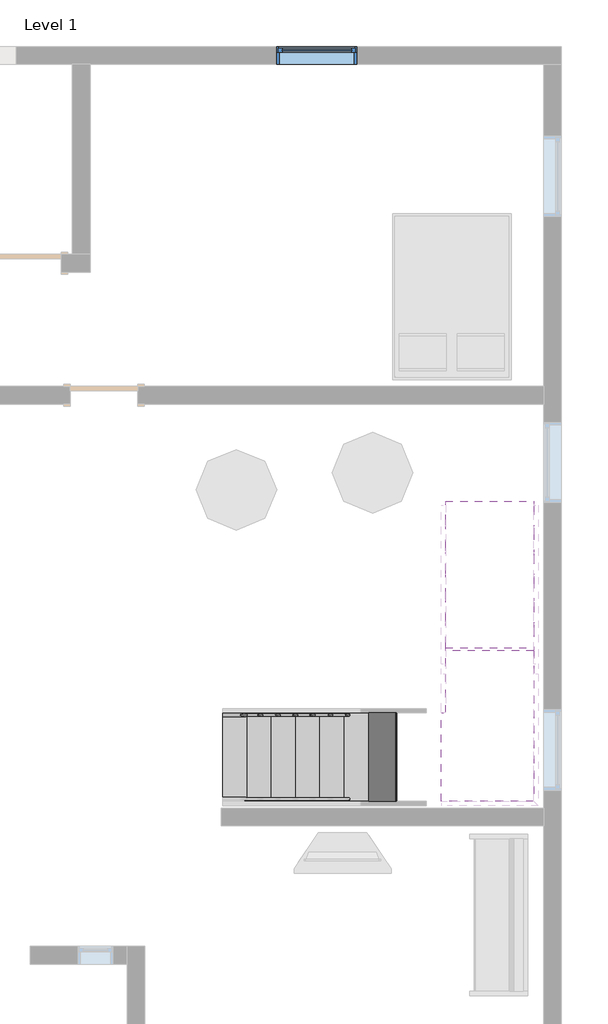
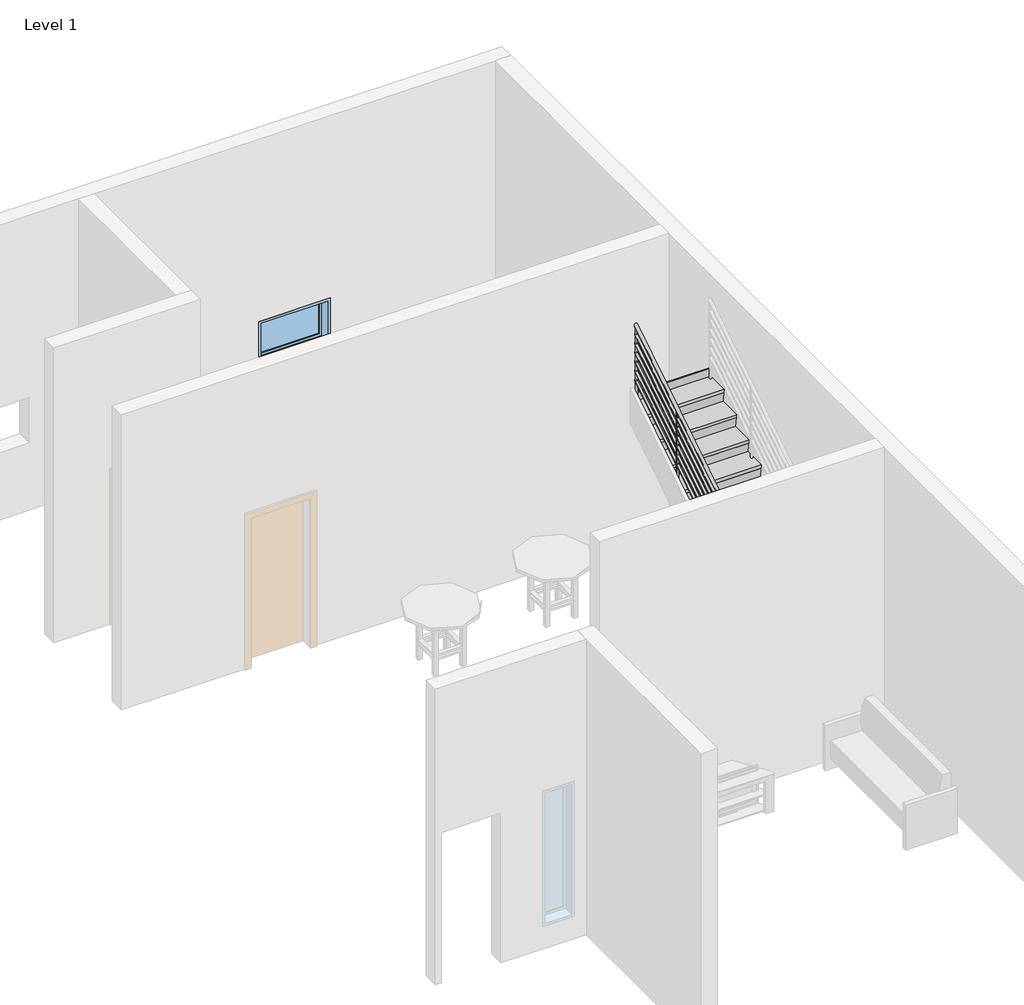
# One storey, part 2 of 4: 2 stair flights, 1 railing, 1 slab, 1 window.
"""IFC4 building model written with IfcOpenShell, lengths in millimetres."""

from ifc_helpers import new_model, si_unit, point, frame, frame_2d, origin, place, context, project, spatial, circle_curve, ellipse_curve, trimmed, segment, composite_curve, outline, extrude, transform, mapped, element, save
from ifc_brep_helpers import plane_surface, cylinder_surface, advanced_brep
from components import non_monolithic_landing_00e8e037, stair_flight_50mm_tread_25mm_nosing_13mm_riser_ecbb9275, stair_flight_50mm_tread_25mm_nosing_13mm_riser_0ce5104d, m_fixed_0915_x_0610mm_70a843a6

model = new_model("IFC4")

# Units and contexts
model_context = context("Model", 3, world=origin())
ifc_project = project(units=[si_unit("LENGTHUNIT", "METRE", prefix="MILLI")], contexts=[model_context])

# Site, building, storey
site = spatial("IfcSite", under=ifc_project)
building = spatial("IfcBuilding", under=site)
storey = spatial("IfcBuildingStorey", under=building, Name="Level 1", Elevation=0.0)

# Railing
placement = place(None, origin())
element("IfcRailing", 1, ObjectType="900mm Pipe", at=placement, inside=storey, context=model_context, shape_type="SolidModel", body=[
    advanced_brep(
    [(-399.786154, 3701.652048, 1050.2491997), (-399.786154, 3741.652048, 1050.2491997), (2081.007299, 3701.652048, 2619.1304348), (2081.007299, 3741.652048, 2619.1304348), (2171.413846, 3701.652048, 2619.1304348), (2131.413846, 3741.652048, 2619.1304348), (2171.413846, 4184.041917, 2619.1304348), (2131.413846, 4184.041917, 2619.1304348), (2171.413846, 6103.248464, 3832.8578953), (2131.413846, 6103.248464, 3832.8578953)],
    [
        (0, 1, ellipse_curve(frame((-399.786154, 3721.652048, 1050.2491997), z_axis=(-1.0, 0.0, 0.0), x_axis=(0.0, 0.0, -1.0)), 23.6638438, 20.0)),
        (1, 0, ellipse_curve(frame((-399.786154, 3721.652048, 1050.2491997), z_axis=(-1.0, 0.0, 0.0), x_axis=(0.0, 0.0, -1.0)), 23.6638438, 20.0)),
        (0, 2),
        (2, 3, ellipse_curve(frame((2081.007299, 3721.652048, 2619.1304348), z_axis=(-0.9605132043335073, 0.0, -0.27823440531497545), x_axis=(0.2782344053149749, 0.0, -0.9605132043335074)), 20.822202, 20.0)),
        (3, 1),
        (3, 2, ellipse_curve(frame((2081.007299, 3721.652048, 2619.1304348), z_axis=(-0.9605132043335073, 0.0, -0.27823440531497545), x_axis=(0.2782344053149749, 0.0, -0.9605132043335074)), 20.822202, 20.0)),
        (2, 4),
        (4, 5, ellipse_curve(frame((2151.413846, 3721.652048, 2619.1304348), z_axis=(-0.7071067811865482, -0.7071067811865468, 0.0), x_axis=(-0.7071067811865468, 0.7071067811865482, 0.0)), 28.2842712, 20.0)),
        (5, 3),
        (5, 4, ellipse_curve(frame((2151.413846, 3721.652048, 2619.1304348), z_axis=(-0.7071067811865482, -0.7071067811865468, 0.0), x_axis=(-0.7071067811865468, 0.7071067811865482, 0.0)), 28.2842712, 20.0)),
        (4, 6),
        (6, 7, ellipse_curve(frame((2151.413846, 4184.041917, 2619.1304348), z_axis=(0.0, -0.9605132043335073, -0.27823440531497556), x_axis=(0.0, -0.2782344053149757, 0.9605132043335073)), 20.822202, 20.0)),
        (7, 5),
        (7, 6, ellipse_curve(frame((2151.413846, 4184.041917, 2619.1304348), z_axis=(0.0, -0.9605132043335073, -0.27823440531497556), x_axis=(0.0, -0.2782344053149757, 0.9605132043335073)), 20.822202, 20.0)),
        (8, 9, ellipse_curve(frame((2151.413846, 6103.248464, 3832.8578953), z_axis=(0.0, 1.0, 0.0), x_axis=(0.0, 0.0, -1.0)), 23.6638438, 20.0)),
        (9, 8, ellipse_curve(frame((2151.413846, 6103.248464, 3832.8578953), z_axis=(0.0, 1.0, 0.0), x_axis=(0.0, 0.0, -1.0)), 23.6638438, 20.0)),
        (6, 8),
        (9, 7),
    ],
    [
        plane_surface(frame((-399.786154, 3721.652048, 1073.9130435), z_axis=(-1.0, 0.0, 0.0), x_axis=(0.0, 1.0, 0.0))),
        cylinder_surface(frame((-389.0962412, 3721.652048, 1057.0096189), z_axis=(-0.845171231398044, 0.0, -0.5344956404098299), x_axis=(0.0, 1.0, 0.0)), 20.0),
        cylinder_surface(frame((2075.213846, 3721.652048, 2619.1304348), z_axis=(-1.0, 0.0, 0.0), x_axis=(0.0, 1.0, 0.0)), 20.0),
        cylinder_surface(frame((2151.413846, 3721.652048, 2619.1304348), z_axis=(0.0, -1.0, 0.0), x_axis=(-1.0, 0.0, 0.0)), 20.0),
        plane_surface(frame((2151.413846, 6103.248464, 3856.5217391), z_axis=(0.0, 1.0, 0.0), x_axis=(0.0, 0.0, 1.0))),
        cylinder_surface(frame((2151.413846, 4188.9383768, 2622.2270102), z_axis=(0.0, -0.8451712313980438, -0.5344956404098301), x_axis=(-1.0, 0.0, 0.0)), 20.0),
    ],
    [
        (0, [[1, 2]]),
        (1, [[-1, 3, 4, 5]]),
        (1, [[-2, -5, 6, -3]]),
        (2, [[-4, 7, 8, 9]]),
        (2, [[-6, -9, 10, -7]]),
        (3, [[-8, 11, 12, 13]]),
        (3, [[-10, -13, 14, -11]]),
        (4, [[15, 16]]),
        (5, [[-12, 17, -16, 18]]),
        (5, [[-14, -18, -15, -17]]),
    ],
),
    advanced_brep(
    [(-399.786154, 3706.652048, 931.1651606), (-399.786154, 3736.652048, 931.1651606), (2079.5589357, 3706.652048, 2499.1304348), (2079.5589357, 3736.652048, 2499.1304348), (2166.413846, 3706.652048, 2499.1304348), (2136.413846, 3736.652048, 2499.1304348), (2166.413846, 4182.5935537, 2499.1304348), (2136.413846, 4182.5935537, 2499.1304348), (2166.413846, 6103.248464, 3713.7738563), (2136.413846, 6103.248464, 3713.7738563)],
    [
        (0, 1, ellipse_curve(frame((-399.786154, 3721.652048, 931.1651606), z_axis=(-1.0, 0.0, 0.0), x_axis=(0.0, 0.0, -1.0)), 17.7478828, 15.0)),
        (1, 0, ellipse_curve(frame((-399.786154, 3721.652048, 931.1651606), z_axis=(-1.0, 0.0, 0.0), x_axis=(0.0, 0.0, -1.0)), 17.7478828, 15.0)),
        (0, 2),
        (2, 3, ellipse_curve(frame((2079.5589357, 3721.652048, 2499.1304348), z_axis=(-0.9605132043335073, 0.0, -0.27823440531497545), x_axis=(0.2782344053149749, 0.0, -0.9605132043335074)), 15.6166515, 15.0)),
        (3, 1),
        (3, 2, ellipse_curve(frame((2079.5589357, 3721.652048, 2499.1304348), z_axis=(-0.9605132043335073, 0.0, -0.27823440531497545), x_axis=(0.2782344053149749, 0.0, -0.9605132043335074)), 15.6166515, 15.0)),
        (2, 4),
        (4, 5, ellipse_curve(frame((2151.413846, 3721.652048, 2499.1304348), z_axis=(-0.7071067811865482, -0.7071067811865468, 0.0), x_axis=(-0.7071067811865468, 0.7071067811865482, 0.0)), 21.2132034, 15.0)),
        (5, 3),
        (5, 4, ellipse_curve(frame((2151.413846, 3721.652048, 2499.1304348), z_axis=(-0.7071067811865482, -0.7071067811865468, 0.0), x_axis=(-0.7071067811865468, 0.7071067811865482, 0.0)), 21.2132034, 15.0)),
        (4, 6),
        (6, 7, ellipse_curve(frame((2151.413846, 4182.5935537, 2499.1304348), z_axis=(0.0, -0.9605132043335073, -0.27823440531497556), x_axis=(0.0, -0.2782344053149757, 0.9605132043335073)), 15.6166515, 15.0)),
        (7, 5),
        (7, 6, ellipse_curve(frame((2151.413846, 4182.5935537, 2499.1304348), z_axis=(0.0, -0.9605132043335073, -0.27823440531497556), x_axis=(0.0, -0.2782344053149757, 0.9605132043335073)), 15.6166515, 15.0)),
        (8, 9, ellipse_curve(frame((2151.413846, 6103.248464, 3713.7738563), z_axis=(0.0, 1.0, 0.0), x_axis=(0.0, 0.0, -1.0)), 17.7478828, 15.0)),
        (9, 8, ellipse_curve(frame((2151.413846, 6103.248464, 3713.7738563), z_axis=(0.0, 1.0, 0.0), x_axis=(0.0, 0.0, -1.0)), 17.7478828, 15.0)),
        (6, 8),
        (9, 7),
    ],
    [
        plane_surface(frame((-399.786154, 3721.652048, 948.9130435), z_axis=(-1.0, 0.0, 0.0), x_axis=(0.0, 1.0, 0.0))),
        cylinder_surface(frame((-391.7687194, 3721.652048, 936.235475), z_axis=(-0.845171231398044, 0.0, -0.5344956404098299), x_axis=(0.0, 1.0, 0.0)), 15.0),
        cylinder_surface(frame((2075.213846, 3721.652048, 2499.1304348), z_axis=(-1.0, 0.0, 0.0), x_axis=(0.0, 1.0, 0.0)), 15.0),
        cylinder_surface(frame((2151.413846, 3721.652048, 2499.1304348), z_axis=(0.0, -1.0, 0.0), x_axis=(-1.0, 0.0, 0.0)), 15.0),
        plane_surface(frame((2151.413846, 6103.248464, 3731.5217391), z_axis=(0.0, 1.0, 0.0), x_axis=(0.0, 0.0, 1.0))),
        cylinder_surface(frame((2151.413846, 4186.2658986, 2501.4528663), z_axis=(0.0, -0.8451712313980438, -0.5344956404098301), x_axis=(-1.0, 0.0, 0.0)), 15.0),
    ],
    [
        (0, [[1, 2]]),
        (1, [[-1, 3, 4, 5]]),
        (1, [[-2, -5, 6, -3]]),
        (2, [[-4, 7, 8, 9]]),
        (2, [[-6, -9, 10, -7]]),
        (3, [[-8, 11, 12, 13]]),
        (3, [[-10, -13, 14, -11]]),
        (4, [[15, 16]]),
        (5, [[-12, 17, -16, 18]]),
        (5, [[-14, -18, -15, -17]]),
    ],
),
    advanced_brep(
    [(-399.786154, 3706.652048, 806.1651606), (-399.786154, 3736.652048, 806.1651606), (2079.5589357, 3706.652048, 2374.1304348), (2079.5589357, 3736.652048, 2374.1304348), (2166.413846, 3706.652048, 2374.1304348), (2136.413846, 3736.652048, 2374.1304348), (2166.413846, 4182.5935537, 2374.1304348), (2136.413846, 4182.5935537, 2374.1304348), (2166.413846, 6103.248464, 3588.7738563), (2136.413846, 6103.248464, 3588.7738563)],
    [
        (0, 1, ellipse_curve(frame((-399.786154, 3721.652048, 806.1651606), z_axis=(-1.0, 0.0, 0.0), x_axis=(0.0, 0.0, -1.0)), 17.7478828, 15.0)),
        (1, 0, ellipse_curve(frame((-399.786154, 3721.652048, 806.1651606), z_axis=(-1.0, 0.0, 0.0), x_axis=(0.0, 0.0, -1.0)), 17.7478828, 15.0)),
        (0, 2),
        (2, 3, ellipse_curve(frame((2079.5589357, 3721.652048, 2374.1304348), z_axis=(-0.9605132043335073, 0.0, -0.27823440531497545), x_axis=(0.2782344053149749, 0.0, -0.9605132043335074)), 15.6166515, 15.0)),
        (3, 1),
        (3, 2, ellipse_curve(frame((2079.5589357, 3721.652048, 2374.1304348), z_axis=(-0.9605132043335073, 0.0, -0.27823440531497545), x_axis=(0.2782344053149749, 0.0, -0.9605132043335074)), 15.6166515, 15.0)),
        (2, 4),
        (4, 5, ellipse_curve(frame((2151.413846, 3721.652048, 2374.1304348), z_axis=(-0.7071067811865482, -0.7071067811865468, 0.0), x_axis=(-0.7071067811865468, 0.7071067811865482, 0.0)), 21.2132034, 15.0)),
        (5, 3),
        (5, 4, ellipse_curve(frame((2151.413846, 3721.652048, 2374.1304348), z_axis=(-0.7071067811865482, -0.7071067811865468, 0.0), x_axis=(-0.7071067811865468, 0.7071067811865482, 0.0)), 21.2132034, 15.0)),
        (4, 6),
        (6, 7, ellipse_curve(frame((2151.413846, 4182.5935537, 2374.1304348), z_axis=(0.0, -0.9605132043335073, -0.27823440531497556), x_axis=(0.0, -0.2782344053149757, 0.9605132043335073)), 15.6166515, 15.0)),
        (7, 5),
        (7, 6, ellipse_curve(frame((2151.413846, 4182.5935537, 2374.1304348), z_axis=(0.0, -0.9605132043335073, -0.27823440531497556), x_axis=(0.0, -0.2782344053149757, 0.9605132043335073)), 15.6166515, 15.0)),
        (8, 9, ellipse_curve(frame((2151.413846, 6103.248464, 3588.7738563), z_axis=(0.0, 1.0, 0.0), x_axis=(0.0, 0.0, -1.0)), 17.7478828, 15.0)),
        (9, 8, ellipse_curve(frame((2151.413846, 6103.248464, 3588.7738563), z_axis=(0.0, 1.0, 0.0), x_axis=(0.0, 0.0, -1.0)), 17.7478828, 15.0)),
        (6, 8),
        (9, 7),
    ],
    [
        plane_surface(frame((-399.786154, 3721.652048, 823.9130435), z_axis=(-1.0, 0.0, 0.0), x_axis=(0.0, 1.0, 0.0))),
        cylinder_surface(frame((-391.7687194, 3721.652048, 811.235475), z_axis=(-0.845171231398044, 0.0, -0.5344956404098299), x_axis=(0.0, 1.0, 0.0)), 15.0),
        cylinder_surface(frame((2075.213846, 3721.652048, 2374.1304348), z_axis=(-1.0, 0.0, 0.0), x_axis=(0.0, 1.0, 0.0)), 15.0),
        cylinder_surface(frame((2151.413846, 3721.652048, 2374.1304348), z_axis=(0.0, -1.0, 0.0), x_axis=(-1.0, 0.0, 0.0)), 15.0),
        plane_surface(frame((2151.413846, 6103.248464, 3606.5217391), z_axis=(0.0, 1.0, 0.0), x_axis=(0.0, 0.0, 1.0))),
        cylinder_surface(frame((2151.413846, 4186.2658986, 2376.4528663), z_axis=(0.0, -0.8451712313980438, -0.5344956404098301), x_axis=(-1.0, 0.0, 0.0)), 15.0),
    ],
    [
        (0, [[1, 2]]),
        (1, [[-1, 3, 4, 5]]),
        (1, [[-2, -5, 6, -3]]),
        (2, [[-4, 7, 8, 9]]),
        (2, [[-6, -9, 10, -7]]),
        (3, [[-8, 11, 12, 13]]),
        (3, [[-10, -13, 14, -11]]),
        (4, [[15, 16]]),
        (5, [[-12, 17, -16, 18]]),
        (5, [[-14, -18, -15, -17]]),
    ],
),
    advanced_brep(
    [(-399.786154, 3706.652048, 681.1651606), (-399.786154, 3736.652048, 681.1651606), (2079.5589357, 3706.652048, 2249.1304348), (2079.5589357, 3736.652048, 2249.1304348), (2166.413846, 3706.652048, 2249.1304348), (2136.413846, 3736.652048, 2249.1304348), (2166.413846, 4182.5935537, 2249.1304348), (2136.413846, 4182.5935537, 2249.1304348), (2166.413846, 6103.248464, 3463.7738563), (2136.413846, 6103.248464, 3463.7738563)],
    [
        (0, 1, ellipse_curve(frame((-399.786154, 3721.652048, 681.1651606), z_axis=(-1.0, 0.0, 0.0), x_axis=(0.0, 0.0, -1.0)), 17.7478828, 15.0)),
        (1, 0, ellipse_curve(frame((-399.786154, 3721.652048, 681.1651606), z_axis=(-1.0, 0.0, 0.0), x_axis=(0.0, 0.0, -1.0)), 17.7478828, 15.0)),
        (0, 2),
        (2, 3, ellipse_curve(frame((2079.5589357, 3721.652048, 2249.1304348), z_axis=(-0.9605132043335073, 0.0, -0.27823440531497545), x_axis=(0.2782344053149749, 0.0, -0.9605132043335074)), 15.6166515, 15.0)),
        (3, 1),
        (3, 2, ellipse_curve(frame((2079.5589357, 3721.652048, 2249.1304348), z_axis=(-0.9605132043335073, 0.0, -0.27823440531497545), x_axis=(0.2782344053149749, 0.0, -0.9605132043335074)), 15.6166515, 15.0)),
        (2, 4),
        (4, 5, ellipse_curve(frame((2151.413846, 3721.652048, 2249.1304348), z_axis=(-0.7071067811865482, -0.7071067811865468, 0.0), x_axis=(-0.7071067811865468, 0.7071067811865482, 0.0)), 21.2132034, 15.0)),
        (5, 3),
        (5, 4, ellipse_curve(frame((2151.413846, 3721.652048, 2249.1304348), z_axis=(-0.7071067811865482, -0.7071067811865468, 0.0), x_axis=(-0.7071067811865468, 0.7071067811865482, 0.0)), 21.2132034, 15.0)),
        (4, 6),
        (6, 7, ellipse_curve(frame((2151.413846, 4182.5935537, 2249.1304348), z_axis=(0.0, -0.9605132043335073, -0.27823440531497545), x_axis=(0.0, -0.2782344053149758, 0.9605132043335072)), 15.6166515, 15.0)),
        (7, 5),
        (7, 6, ellipse_curve(frame((2151.413846, 4182.5935537, 2249.1304348), z_axis=(0.0, -0.9605132043335073, -0.27823440531497545), x_axis=(0.0, -0.2782344053149758, 0.9605132043335072)), 15.6166515, 15.0)),
        (8, 9, ellipse_curve(frame((2151.413846, 6103.248464, 3463.7738563), z_axis=(0.0, 1.0, 0.0), x_axis=(0.0, 0.0, -1.0)), 17.7478828, 15.0)),
        (9, 8, ellipse_curve(frame((2151.413846, 6103.248464, 3463.7738563), z_axis=(0.0, 1.0, 0.0), x_axis=(0.0, 0.0, -1.0)), 17.7478828, 15.0)),
        (6, 8),
        (9, 7),
    ],
    [
        plane_surface(frame((-399.786154, 3721.652048, 698.9130435), z_axis=(-1.0, 0.0, 0.0), x_axis=(0.0, 1.0, 0.0))),
        cylinder_surface(frame((-391.7687194, 3721.652048, 686.235475), z_axis=(-0.845171231398044, 0.0, -0.5344956404098299), x_axis=(0.0, 1.0, 0.0)), 15.0),
        cylinder_surface(frame((2075.213846, 3721.652048, 2249.1304348), z_axis=(-1.0, 0.0, 0.0), x_axis=(0.0, 1.0, 0.0)), 15.0),
        cylinder_surface(frame((2151.413846, 3721.652048, 2249.1304348), z_axis=(0.0, -1.0, 0.0), x_axis=(-1.0, 0.0, 0.0)), 15.0),
        plane_surface(frame((2151.413846, 6103.248464, 3481.5217391), z_axis=(0.0, 1.0, 0.0), x_axis=(0.0, 0.0, 1.0))),
        cylinder_surface(frame((2151.413846, 4186.2658986, 2251.4528663), z_axis=(0.0, -0.845171231398044, -0.5344956404098299), x_axis=(-1.0, 0.0, 0.0)), 15.0),
    ],
    [
        (0, [[1, 2]]),
        (1, [[-1, 3, 4, 5]]),
        (1, [[-2, -5, 6, -3]]),
        (2, [[-4, 7, 8, 9]]),
        (2, [[-6, -9, 10, -7]]),
        (3, [[-8, 11, 12, 13]]),
        (3, [[-10, -13, 14, -11]]),
        (4, [[15, 16]]),
        (5, [[-12, 17, -16, 18]]),
        (5, [[-14, -18, -15, -17]]),
    ],
),
    advanced_brep(
    [(-399.786154, 3706.652048, 556.1651606), (-399.786154, 3736.652048, 556.1651606), (2079.5589357, 3706.652048, 2124.1304348), (2079.5589357, 3736.652048, 2124.1304348), (2166.413846, 3706.652048, 2124.1304348), (2136.413846, 3736.652048, 2124.1304348), (2166.413846, 4182.5935537, 2124.1304348), (2136.413846, 4182.5935537, 2124.1304348), (2166.413846, 6103.248464, 3338.7738563), (2136.413846, 6103.248464, 3338.7738563)],
    [
        (0, 1, ellipse_curve(frame((-399.786154, 3721.652048, 556.1651606), z_axis=(-1.0, 0.0, 0.0), x_axis=(0.0, 0.0, -1.0)), 17.7478828, 15.0)),
        (1, 0, ellipse_curve(frame((-399.786154, 3721.652048, 556.1651606), z_axis=(-1.0, 0.0, 0.0), x_axis=(0.0, 0.0, -1.0)), 17.7478828, 15.0)),
        (0, 2),
        (2, 3, ellipse_curve(frame((2079.5589357, 3721.652048, 2124.1304348), z_axis=(-0.9605132043335073, 0.0, -0.27823440531497545), x_axis=(0.2782344053149749, 0.0, -0.9605132043335074)), 15.6166515, 15.0)),
        (3, 1),
        (3, 2, ellipse_curve(frame((2079.5589357, 3721.652048, 2124.1304348), z_axis=(-0.9605132043335073, 0.0, -0.27823440531497545), x_axis=(0.2782344053149749, 0.0, -0.9605132043335074)), 15.6166515, 15.0)),
        (2, 4),
        (4, 5, ellipse_curve(frame((2151.413846, 3721.652048, 2124.1304348), z_axis=(-0.7071067811865482, -0.7071067811865468, 0.0), x_axis=(-0.7071067811865468, 0.7071067811865482, 0.0)), 21.2132034, 15.0)),
        (5, 3),
        (5, 4, ellipse_curve(frame((2151.413846, 3721.652048, 2124.1304348), z_axis=(-0.7071067811865482, -0.7071067811865468, 0.0), x_axis=(-0.7071067811865468, 0.7071067811865482, 0.0)), 21.2132034, 15.0)),
        (4, 6),
        (6, 7, ellipse_curve(frame((2151.413846, 4182.5935537, 2124.1304348), z_axis=(0.0, -0.9605132043335073, -0.27823440531497556), x_axis=(0.0, -0.2782344053149757, 0.9605132043335073)), 15.6166515, 15.0)),
        (7, 5),
        (7, 6, ellipse_curve(frame((2151.413846, 4182.5935537, 2124.1304348), z_axis=(0.0, -0.9605132043335073, -0.27823440531497556), x_axis=(0.0, -0.2782344053149757, 0.9605132043335073)), 15.6166515, 15.0)),
        (8, 9, ellipse_curve(frame((2151.413846, 6103.248464, 3338.7738563), z_axis=(0.0, 1.0, 0.0), x_axis=(0.0, 0.0, -1.0)), 17.7478828, 15.0)),
        (9, 8, ellipse_curve(frame((2151.413846, 6103.248464, 3338.7738563), z_axis=(0.0, 1.0, 0.0), x_axis=(0.0, 0.0, -1.0)), 17.7478828, 15.0)),
        (6, 8),
        (9, 7),
    ],
    [
        plane_surface(frame((-399.786154, 3721.652048, 573.9130435), z_axis=(-1.0, 0.0, 0.0), x_axis=(0.0, 1.0, 0.0))),
        cylinder_surface(frame((-391.7687194, 3721.652048, 561.235475), z_axis=(-0.845171231398044, 0.0, -0.5344956404098299), x_axis=(0.0, 1.0, 0.0)), 15.0),
        cylinder_surface(frame((2075.213846, 3721.652048, 2124.1304348), z_axis=(-1.0, 0.0, 0.0), x_axis=(0.0, 1.0, 0.0)), 15.0),
        cylinder_surface(frame((2151.413846, 3721.652048, 2124.1304348), z_axis=(0.0, -1.0, 0.0), x_axis=(-1.0, 0.0, 0.0)), 15.0),
        plane_surface(frame((2151.413846, 6103.248464, 3356.5217391), z_axis=(0.0, 1.0, 0.0), x_axis=(0.0, 0.0, 1.0))),
        cylinder_surface(frame((2151.413846, 4186.2658986, 2126.4528663), z_axis=(0.0, -0.8451712313980438, -0.5344956404098301), x_axis=(-1.0, 0.0, 0.0)), 15.0),
    ],
    [
        (0, [[1, 2]]),
        (1, [[-1, 3, 4, 5]]),
        (1, [[-2, -5, 6, -3]]),
        (2, [[-4, 7, 8, 9]]),
        (2, [[-6, -9, 10, -7]]),
        (3, [[-8, 11, 12, 13]]),
        (3, [[-10, -13, 14, -11]]),
        (4, [[15, 16]]),
        (5, [[-12, 17, -16, 18]]),
        (5, [[-14, -18, -15, -17]]),
    ],
),
    advanced_brep(
    [(-399.786154, 3706.652048, 431.1651606), (-399.786154, 3736.652048, 431.1651606), (2079.5589357, 3706.652048, 1999.1304348), (2079.5589357, 3736.652048, 1999.1304348), (2166.413846, 3706.652048, 1999.1304348), (2136.413846, 3736.652048, 1999.1304348), (2166.413846, 4182.5935537, 1999.1304348), (2136.413846, 4182.5935537, 1999.1304348), (2166.413846, 6103.248464, 3213.7738563), (2136.413846, 6103.248464, 3213.7738563)],
    [
        (0, 1, ellipse_curve(frame((-399.786154, 3721.652048, 431.1651606), z_axis=(-1.0, 0.0, 0.0), x_axis=(0.0, 0.0, -1.0)), 17.7478828, 15.0)),
        (1, 0, ellipse_curve(frame((-399.786154, 3721.652048, 431.1651606), z_axis=(-1.0, 0.0, 0.0), x_axis=(0.0, 0.0, -1.0)), 17.7478828, 15.0)),
        (0, 2),
        (2, 3, ellipse_curve(frame((2079.5589357, 3721.652048, 1999.1304348), z_axis=(-0.9605132043335073, 0.0, -0.27823440531497545), x_axis=(0.2782344053149749, 0.0, -0.9605132043335074)), 15.6166515, 15.0)),
        (3, 1),
        (3, 2, ellipse_curve(frame((2079.5589357, 3721.652048, 1999.1304348), z_axis=(-0.9605132043335073, 0.0, -0.27823440531497545), x_axis=(0.2782344053149749, 0.0, -0.9605132043335074)), 15.6166515, 15.0)),
        (2, 4),
        (4, 5, ellipse_curve(frame((2151.413846, 3721.652048, 1999.1304348), z_axis=(-0.7071067811865482, -0.7071067811865468, 0.0), x_axis=(-0.7071067811865468, 0.7071067811865482, 0.0)), 21.2132034, 15.0)),
        (5, 3),
        (5, 4, ellipse_curve(frame((2151.413846, 3721.652048, 1999.1304348), z_axis=(-0.7071067811865482, -0.7071067811865468, 0.0), x_axis=(-0.7071067811865468, 0.7071067811865482, 0.0)), 21.2132034, 15.0)),
        (4, 6),
        (6, 7, ellipse_curve(frame((2151.413846, 4182.5935537, 1999.1304348), z_axis=(0.0, -0.9605132043335072, -0.27823440531497556), x_axis=(0.0, -0.27823440531497606, 0.9605132043335073)), 15.6166515, 15.0)),
        (7, 5),
        (7, 6, ellipse_curve(frame((2151.413846, 4182.5935537, 1999.1304348), z_axis=(0.0, -0.9605132043335072, -0.27823440531497556), x_axis=(0.0, -0.27823440531497606, 0.9605132043335073)), 15.6166515, 15.0)),
        (8, 9, ellipse_curve(frame((2151.413846, 6103.248464, 3213.7738563), z_axis=(0.0, 1.0, 0.0), x_axis=(0.0, 0.0, -1.0)), 17.7478828, 15.0)),
        (9, 8, ellipse_curve(frame((2151.413846, 6103.248464, 3213.7738563), z_axis=(0.0, 1.0, 0.0), x_axis=(0.0, 0.0, -1.0)), 17.7478828, 15.0)),
        (6, 8),
        (9, 7),
    ],
    [
        plane_surface(frame((-399.786154, 3721.652048, 448.9130435), z_axis=(-1.0, 0.0, 0.0), x_axis=(0.0, 1.0, 0.0))),
        cylinder_surface(frame((-391.7687194, 3721.652048, 436.235475), z_axis=(-0.845171231398044, 0.0, -0.5344956404098299), x_axis=(0.0, 1.0, 0.0)), 15.0),
        cylinder_surface(frame((2075.213846, 3721.652048, 1999.1304348), z_axis=(-1.0, 0.0, 0.0), x_axis=(0.0, 1.0, 0.0)), 15.0),
        cylinder_surface(frame((2151.413846, 3721.652048, 1999.1304348), z_axis=(0.0, -1.0, 0.0), x_axis=(-1.0, 0.0, 0.0)), 15.0),
        plane_surface(frame((2151.413846, 6103.248464, 3231.5217391), z_axis=(0.0, 1.0, 0.0), x_axis=(0.0, 0.0, 1.0))),
        cylinder_surface(frame((2151.413846, 4186.2658986, 2001.4528663), z_axis=(0.0, -0.8451712313980437, -0.5344956404098301), x_axis=(-1.0, 0.0, 0.0)), 15.0),
    ],
    [
        (0, [[1, 2]]),
        (1, [[-1, 3, 4, 5]]),
        (1, [[-2, -5, 6, -3]]),
        (2, [[-4, 7, 8, 9]]),
        (2, [[-6, -9, 10, -7]]),
        (3, [[-8, 11, 12, 13]]),
        (3, [[-10, -13, 14, -11]]),
        (4, [[15, 16]]),
        (5, [[-12, 17, -16, 18]]),
        (5, [[-14, -18, -15, -17]]),
    ],
),
    advanced_brep(
    [(-399.786154, 3706.652048, 306.1651606), (-399.786154, 3736.652048, 306.1651606), (2079.5589357, 3706.652048, 1874.1304348), (2079.5589357, 3736.652048, 1874.1304348), (2166.413846, 3706.652048, 1874.1304348), (2136.413846, 3736.652048, 1874.1304348), (2166.413846, 4182.5935537, 1874.1304348), (2136.413846, 4182.5935537, 1874.1304348), (2166.413846, 6103.248464, 3088.7738563), (2136.413846, 6103.248464, 3088.7738563)],
    [
        (0, 1, ellipse_curve(frame((-399.786154, 3721.652048, 306.1651606), z_axis=(-1.0, 0.0, 0.0), x_axis=(0.0, 0.0, -1.0)), 17.7478828, 15.0)),
        (1, 0, ellipse_curve(frame((-399.786154, 3721.652048, 306.1651606), z_axis=(-1.0, 0.0, 0.0), x_axis=(0.0, 0.0, -1.0)), 17.7478828, 15.0)),
        (0, 2),
        (2, 3, ellipse_curve(frame((2079.5589357, 3721.652048, 1874.1304348), z_axis=(-0.9605132043335073, 0.0, -0.27823440531497545), x_axis=(0.2782344053149749, 0.0, -0.9605132043335074)), 15.6166515, 15.0)),
        (3, 1),
        (3, 2, ellipse_curve(frame((2079.5589357, 3721.652048, 1874.1304348), z_axis=(-0.9605132043335073, 0.0, -0.27823440531497545), x_axis=(0.2782344053149749, 0.0, -0.9605132043335074)), 15.6166515, 15.0)),
        (2, 4),
        (4, 5, ellipse_curve(frame((2151.413846, 3721.652048, 1874.1304348), z_axis=(-0.7071067811865482, -0.7071067811865468, 0.0), x_axis=(-0.7071067811865468, 0.7071067811865482, 0.0)), 21.2132034, 15.0)),
        (5, 3),
        (5, 4, ellipse_curve(frame((2151.413846, 3721.652048, 1874.1304348), z_axis=(-0.7071067811865482, -0.7071067811865468, 0.0), x_axis=(-0.7071067811865468, 0.7071067811865482, 0.0)), 21.2132034, 15.0)),
        (4, 6),
        (6, 7, ellipse_curve(frame((2151.413846, 4182.5935537, 1874.1304348), z_axis=(0.0, -0.9605132043335073, -0.27823440531497556), x_axis=(0.0, -0.2782344053149757, 0.9605132043335073)), 15.6166515, 15.0)),
        (7, 5),
        (7, 6, ellipse_curve(frame((2151.413846, 4182.5935537, 1874.1304348), z_axis=(0.0, -0.9605132043335073, -0.27823440531497556), x_axis=(0.0, -0.2782344053149757, 0.9605132043335073)), 15.6166515, 15.0)),
        (8, 9, ellipse_curve(frame((2151.413846, 6103.248464, 3088.7738563), z_axis=(0.0, 1.0, 0.0), x_axis=(0.0, 0.0, -1.0)), 17.7478828, 15.0)),
        (9, 8, ellipse_curve(frame((2151.413846, 6103.248464, 3088.7738563), z_axis=(0.0, 1.0, 0.0), x_axis=(0.0, 0.0, -1.0)), 17.7478828, 15.0)),
        (6, 8),
        (9, 7),
    ],
    [
        plane_surface(frame((-399.786154, 3721.652048, 323.9130435), z_axis=(-1.0, 0.0, 0.0), x_axis=(0.0, 1.0, 0.0))),
        cylinder_surface(frame((-391.7687194, 3721.652048, 311.235475), z_axis=(-0.845171231398044, 0.0, -0.5344956404098299), x_axis=(0.0, 1.0, 0.0)), 15.0),
        cylinder_surface(frame((2075.213846, 3721.652048, 1874.1304348), z_axis=(-1.0, 0.0, 0.0), x_axis=(0.0, 1.0, 0.0)), 15.0),
        cylinder_surface(frame((2151.413846, 3721.652048, 1874.1304348), z_axis=(0.0, -1.0, 0.0), x_axis=(-1.0, 0.0, 0.0)), 15.0),
        plane_surface(frame((2151.413846, 6103.248464, 3106.5217391), z_axis=(0.0, 1.0, 0.0), x_axis=(0.0, 0.0, 1.0))),
        cylinder_surface(frame((2151.413846, 4186.2658986, 1876.4528663), z_axis=(0.0, -0.8451712313980438, -0.5344956404098301), x_axis=(-1.0, 0.0, 0.0)), 15.0),
    ],
    [
        (0, [[1, 2]]),
        (1, [[-1, 3, 4, 5]]),
        (1, [[-2, -5, 6, -3]]),
        (2, [[-4, 7, 8, 9]]),
        (2, [[-6, -9, 10, -7]]),
        (3, [[-8, 11, 12, 13]]),
        (3, [[-10, -13, 14, -11]]),
        (4, [[15, 16]]),
        (5, [[-12, 17, -16, 18]]),
        (5, [[-14, -18, -15, -17]]),
    ],
),
    advanced_brep(
    [(2138.913846, 5178.248464, 3224.2138144), (2163.913846, 5178.248464, 3224.2138144), (2163.913846, 5178.248464, 2260.8695652), (2138.913846, 5178.248464, 2260.8695652)],
    [
        (0, 1, ellipse_curve(frame((2151.413846, 5178.248464, 3224.2138144), z_axis=(0.0, 0.5344956404098302, -0.8451712313980437), x_axis=(0.0, 0.8451712313980437, 0.53449564040983)), 14.7899024, 12.5)),
        (1, 2),
        (2, 3, circle_curve(frame((2151.413846, 5178.248464, 2260.8695652), z_axis=(0.0, 0.0, 1.0), x_axis=(1.0, 0.0, 0.0)), 12.5)),
        (3, 0),
        (3, 2, circle_curve(frame((2151.413846, 5178.248464, 2260.8695652), z_axis=(0.0, 0.0, 1.0), x_axis=(1.0, 0.0, 0.0)), 12.5)),
        (1, 0, ellipse_curve(frame((2151.413846, 5178.248464, 3224.2138144), z_axis=(0.0, 0.5344956404098302, -0.8451712313980437), x_axis=(0.0, 0.8451712313980437, 0.53449564040983)), 14.7899024, 12.5)),
    ],
    [
        cylinder_surface(frame((2151.413846, 5178.248464, 2160.8695652), z_axis=(0.0, 0.0, 1.0), x_axis=(1.0, 0.0, 0.0)), 12.5),
        plane_surface(frame((2176.413846, 5203.248464, 3240.0240911), z_axis=(0.0, -0.5344956404098302, 0.8451712313980437), x_axis=(-1.0, 0.0, 0.0))),
        plane_surface(frame((2176.413846, 5153.248464, 2260.8695652), z_axis=(0.0, 0.0, -1.0), x_axis=(-1.0, 0.0, 0.0))),
    ],
    [
        (0, [[1, 2, 3, 4]]),
        (0, [[5, -2, 6, -4]]),
        (1, [[-6, -1]]),
        (2, [[-5, -3]]),
    ],
),
    advanced_brep(
    [(1600.213846, 3734.152048, 2291.4074903), (1600.213846, 3709.152048, 2291.4074903), (1600.213846, 3709.152048, 1391.3043478), (1600.213846, 3734.152048, 1391.3043478)],
    [
        (0, 1, ellipse_curve(frame((1600.213846, 3721.652048, 2291.4074903), z_axis=(0.5344956404098302, 0.0, -0.8451712313980437), x_axis=(0.8451712313980437, 0.0, 0.53449564040983)), 14.7899024, 12.5)),
        (1, 2),
        (2, 3, circle_curve(frame((1600.213846, 3721.652048, 1391.3043478), z_axis=(0.0, 0.0, 1.0), x_axis=(0.0, -1.0, 0.0)), 12.5)),
        (3, 0),
        (3, 2, circle_curve(frame((1600.213846, 3721.652048, 1391.3043478), z_axis=(0.0, 0.0, 1.0), x_axis=(0.0, -1.0, 0.0)), 12.5)),
        (1, 0, ellipse_curve(frame((1600.213846, 3721.652048, 2291.4074903), z_axis=(0.5344956404098302, 0.0, -0.8451712313980437), x_axis=(0.8451712313980437, 0.0, 0.53449564040983)), 14.7899024, 12.5)),
    ],
    [
        cylinder_surface(frame((1600.213846, 3721.652048, 1291.3043478), z_axis=(0.0, 0.0, 1.0), x_axis=(0.0, -1.0, 0.0)), 12.5),
        plane_surface(frame((1625.213846, 3696.652048, 2307.217767), z_axis=(-0.5344956404098302, 0.0, 0.8451712313980437), x_axis=(0.0, 1.0, 0.0))),
        plane_surface(frame((1575.213846, 3696.652048, 1391.3043478), z_axis=(0.0, 0.0, -1.0), x_axis=(0.0, 1.0, 0.0))),
    ],
    [
        (0, [[1, 2, 3, 4]]),
        (0, [[5, -2, 6, -4]]),
        (1, [[-6, -1]]),
        (2, [[-5, -3]]),
    ],
),
    advanced_brep(
    [(600.213846, 3734.152048, 1658.9964231), (600.213846, 3709.152048, 1658.9964231), (600.213846, 3709.152048, 695.6521739), (600.213846, 3734.152048, 695.6521739)],
    [
        (0, 1, ellipse_curve(frame((600.213846, 3721.652048, 1658.9964231), z_axis=(0.5344956404098302, 0.0, -0.8451712313980437), x_axis=(0.8451712313980437, 0.0, 0.53449564040983)), 14.7899024, 12.5)),
        (1, 2),
        (2, 3, circle_curve(frame((600.213846, 3721.652048, 695.6521739), z_axis=(0.0, 0.0, 1.0), x_axis=(0.0, -1.0, 0.0)), 12.5)),
        (3, 0),
        (3, 2, circle_curve(frame((600.213846, 3721.652048, 695.6521739), z_axis=(0.0, 0.0, 1.0), x_axis=(0.0, -1.0, 0.0)), 12.5)),
        (1, 0, ellipse_curve(frame((600.213846, 3721.652048, 1658.9964231), z_axis=(0.5344956404098302, 0.0, -0.8451712313980437), x_axis=(0.8451712313980437, 0.0, 0.53449564040983)), 14.7899024, 12.5)),
    ],
    [
        cylinder_surface(frame((600.213846, 3721.652048, 595.6521739), z_axis=(0.0, 0.0, 1.0), x_axis=(0.0, -1.0, 0.0)), 12.5),
        plane_surface(frame((625.213846, 3696.652048, 1674.8066998), z_axis=(-0.5344956404098302, 0.0, 0.8451712313980437), x_axis=(0.0, 1.0, 0.0))),
        plane_surface(frame((575.213846, 3696.652048, 695.6521739), z_axis=(0.0, 0.0, -1.0), x_axis=(0.0, 1.0, 0.0))),
    ],
    [
        (0, [[1, 2, 3, 4]]),
        (0, [[5, -2, 6, -4]]),
        (1, [[-6, -1]]),
        (2, [[-5, -3]]),
    ],
),
    extrude(outline(composite_curve([segment(trimmed(circle_curve(frame_2d((2151.413846, 4178.248464)), 12.5), [point((2163.913846, 4178.248464))], [point((2138.913846, 4178.248464))], False, "CARTESIAN"), True, "CONTINUOUS"), segment(trimmed(circle_curve(frame_2d((2151.413846, 4178.248464)), 12.5), [point((2138.913846, 4178.248464))], [point((2163.913846, 4178.248464))], False, "CARTESIAN"), True, "CONTINUOUS")], self_intersect=False)), frame((0.0, 0.0, 1739.1304348), z_axis=(0.0, 0.0, 1.0), x_axis=(1.0, 0.0, 0.0)), (0.0, 0.0, 1.0), 860.0),
    extrude(outline(composite_curve([segment(trimmed(circle_curve(frame_2d((2151.413846, 3721.652048)), 12.5), [point((2151.413846, 3709.152048))], [point((2151.413846, 3734.152048))], False, "CARTESIAN"), True, "CONTINUOUS"), segment(trimmed(circle_curve(frame_2d((2151.413846, 3721.652048)), 12.5), [point((2151.413846, 3734.152048))], [point((2151.413846, 3709.152048))], False, "CARTESIAN"), True, "CONTINUOUS")], self_intersect=False)), frame((0.0, 0.0, 1739.1304348), z_axis=(0.0, 0.0, 1.0), x_axis=(1.0, 0.0, 0.0)), (0.0, 0.0, 1.0), 860.0),
    advanced_brep(
    [(2075.213846, 3734.152048, 2591.8027472), (2075.213846, 3709.152048, 2591.8027472), (2075.213846, 3709.152048, 1739.1304348), (2075.213846, 3734.152048, 1739.1304348)],
    [
        (0, 1, ellipse_curve(frame((2075.213846, 3721.652048, 2591.8027472), z_axis=(0.5344956404098302, 0.0, -0.8451712313980437), x_axis=(0.8451712313980437, 0.0, 0.53449564040983)), 14.7899024, 12.5)),
        (1, 2),
        (2, 3, circle_curve(frame((2075.213846, 3721.652048, 1739.1304348), z_axis=(0.0, 0.0, 1.0), x_axis=(0.0, -1.0, 0.0)), 12.5)),
        (3, 0),
        (3, 2, circle_curve(frame((2075.213846, 3721.652048, 1739.1304348), z_axis=(0.0, 0.0, 1.0), x_axis=(0.0, -1.0, 0.0)), 12.5)),
        (1, 0, ellipse_curve(frame((2075.213846, 3721.652048, 2591.8027472), z_axis=(0.5344956404098302, 0.0, -0.8451712313980437), x_axis=(0.8451712313980437, 0.0, 0.53449564040983)), 14.7899024, 12.5)),
    ],
    [
        cylinder_surface(frame((2075.213846, 3721.652048, 1639.1304348), z_axis=(0.0, 0.0, 1.0), x_axis=(0.0, -1.0, 0.0)), 12.5),
        plane_surface(frame((2100.213846, 3696.652048, 2607.6130239), z_axis=(-0.5344956404098302, 0.0, 0.8451712313980437), x_axis=(0.0, 1.0, 0.0))),
        plane_surface(frame((2050.213846, 3696.652048, 1739.1304348), z_axis=(0.0, 0.0, -1.0), x_axis=(0.0, 1.0, 0.0))),
    ],
    [
        (0, [[1, 2, 3, 4]]),
        (0, [[5, -2, 6, -4]]),
        (1, [[-6, -1]]),
        (2, [[-5, -3]]),
    ],
),
    advanced_brep(
    [(2138.913846, 6090.748464, 3801.2889132), (2163.913846, 6090.748464, 3801.2889132), (2163.913846, 6090.748464, 2782.6086957), (2138.913846, 6090.748464, 2782.6086957)],
    [
        (0, 1, ellipse_curve(frame((2151.413846, 6090.748464, 3801.2889132), z_axis=(0.0, 0.5344956404098302, -0.8451712313980437), x_axis=(0.0, 0.8451712313980437, 0.53449564040983)), 14.7899024, 12.5)),
        (1, 2),
        (2, 3, circle_curve(frame((2151.413846, 6090.748464, 2782.6086957), z_axis=(0.0, 0.0, 1.0), x_axis=(1.0, 0.0, 0.0)), 12.5)),
        (3, 0),
        (3, 2, circle_curve(frame((2151.413846, 6090.748464, 2782.6086957), z_axis=(0.0, 0.0, 1.0), x_axis=(1.0, 0.0, 0.0)), 12.5)),
        (1, 0, ellipse_curve(frame((2151.413846, 6090.748464, 3801.2889132), z_axis=(0.0, 0.5344956404098302, -0.8451712313980437), x_axis=(0.0, 0.8451712313980437, 0.53449564040983)), 14.7899024, 12.5)),
    ],
    [
        cylinder_surface(frame((2151.413846, 6090.748464, 2682.6086957), z_axis=(0.0, 0.0, 1.0), x_axis=(1.0, 0.0, 0.0)), 12.5),
        plane_surface(frame((2176.413846, 6115.748464, 3817.0991899), z_axis=(0.0, -0.5344956404098302, 0.8451712313980437), x_axis=(-1.0, 0.0, 0.0))),
        plane_surface(frame((2176.413846, 6065.748464, 2782.6086957), z_axis=(0.0, 0.0, -1.0), x_axis=(-1.0, 0.0, 0.0))),
    ],
    [
        (0, [[1, 2, 3, 4]]),
        (0, [[5, -2, 6, -4]]),
        (1, [[-6, -1]]),
        (2, [[-5, -3]]),
    ],
),
    advanced_brep(
    [(-387.286154, 3734.152048, 1034.4904942), (-387.286154, 3709.152048, 1034.4904942), (-387.286154, 3709.152048, 173.9130435), (-387.286154, 3734.152048, 173.9130435)],
    [
        (0, 1, ellipse_curve(frame((-387.286154, 3721.652048, 1034.4904942), z_axis=(0.5344956404098302, 0.0, -0.8451712313980437), x_axis=(0.8451712313980437, 0.0, 0.53449564040983)), 14.7899024, 12.5)),
        (1, 2),
        (2, 3, circle_curve(frame((-387.286154, 3721.652048, 173.9130435), z_axis=(0.0, 0.0, 1.0), x_axis=(0.0, -1.0, 0.0)), 12.5)),
        (3, 0),
        (3, 2, circle_curve(frame((-387.286154, 3721.652048, 173.9130435), z_axis=(0.0, 0.0, 1.0), x_axis=(0.0, -1.0, 0.0)), 12.5)),
        (1, 0, ellipse_curve(frame((-387.286154, 3721.652048, 1034.4904942), z_axis=(0.5344956404098302, 0.0, -0.8451712313980437), x_axis=(0.8451712313980437, 0.0, 0.53449564040983)), 14.7899024, 12.5)),
    ],
    [
        cylinder_surface(frame((-387.286154, 3721.652048, 73.9130435), z_axis=(0.0, 0.0, 1.0), x_axis=(0.0, -1.0, 0.0)), 12.5),
        plane_surface(frame((-362.286154, 3696.652048, 1050.3007709), z_axis=(-0.5344956404098302, 0.0, 0.8451712313980437), x_axis=(0.0, 1.0, 0.0))),
        plane_surface(frame((-412.286154, 3696.652048, 173.9130435), z_axis=(0.0, 0.0, -1.0), x_axis=(0.0, 1.0, 0.0))),
    ],
    [
        (0, [[1, 2, 3, 4]]),
        (0, [[5, -2, 6, -4]]),
        (1, [[-6, -1]]),
        (2, [[-5, -3]]),
    ],
),
])

# Slab
non_monolithic_landing_shape = non_monolithic_landing_00e8e037(model_context)
element("IfcSlab", 2, ObjectType="Non-Monolithic Landing", at=placement, inside=storey, context=model_context, shape_type="MappedRepresentation", body=[
    mapped(non_monolithic_landing_shape, transform((0.0, 0.0, 0.0), x_axis=(1.0, 0.0, 0.0), y_axis=(0.0, 1.0, 0.0), z_axis=(0.0, 0.0, 1.0))),
])

# Stair flights
stair_flight_50mm_tread_25mm_nosing_13mm_riser_shape = stair_flight_50mm_tread_25mm_nosing_13mm_riser_ecbb9275(model_context)
element("IfcStairFlight", 3, ObjectType="50mm Tread 25mm Nosing 13mm Riser", at=placement, inside=storey, context=model_context, shape_type="MappedRepresentation", body=[
    mapped(stair_flight_50mm_tread_25mm_nosing_13mm_riser_shape, transform((0.0, 0.0, 0.0), x_axis=(1.0, 0.0, 0.0), y_axis=(0.0, 1.0, 0.0), z_axis=(0.0, 0.0, 1.0))),
])
stair_flight_50mm_tread_25mm_nosing_13mm_riser_2_shape = stair_flight_50mm_tread_25mm_nosing_13mm_riser_0ce5104d(model_context)
element("IfcStairFlight", 4, ObjectType="50mm Tread 25mm Nosing 13mm Riser", at=placement, inside=storey, context=model_context, shape_type="MappedRepresentation", body=[
    mapped(stair_flight_50mm_tread_25mm_nosing_13mm_riser_2_shape, transform((0.0, 0.0, 0.0), x_axis=(1.0, 0.0, 0.0), y_axis=(0.0, 1.0, 0.0), z_axis=(0.0, 0.0, 1.0))),
])

# Window
m_fixed_0915_x_0610mm_shape = m_fixed_0915_x_0610mm_70a843a6(model_context)
element("IfcWindow", 5, ObjectType="M_Fixed : 0915 x 0610mm", at=placement, inside=storey, context=model_context, shape_type="MappedRepresentation", body=[
    mapped(m_fixed_0915_x_0610mm_shape, transform((665.4267366, 11191.848464, 0.0), x_axis=(1.0, 0.0, 0.0), y_axis=(0.0, 1.0, 0.0), z_axis=(0.0, 0.0, 1.0))),
])

save(model, "model.ifc")

# Revit data of these elements
# Type "900mm Pipe"
#   built-in parameter 1008612 = 0.019685 (stored number, unit not read)
#   built-in parameter 1008611 = 0.0984252 (stored number, unit not read)
#   built-in parameter 1008609 = 6.56168 (stored number, unit not read)
#   built-in parameter 1008604 = 0.19685 (stored number, unit not read)
#   built-in parameter 1008603 = 0.164042 (stored number, unit not read)
#   Railing Height = 2' - 11.43307"
#   built-in parameter 1008630 = 2
#   built-in parameter 1008610 = 2
#   built-in parameter 1008605 = 1
#   built-in parameter 1008618 = M_Baluster - Round : 25mm
# Type "M_Fixed : 0915 x 0610mm"
#   Type Mark = "14"
#   Height = 2' - 0.01575"
#   Default Sill Height = 3' - 0.02362"
#   Width = 3' - 0.02362"
#   Window Inset = 0' - 0.74803"
#   Frame Exterior Material = Sash
#   Frame Interior Material = Sash
#   Glass Pane Material = Glass
#   Sash = Sash
#   Wall Closure = (empty or 0)
# Element 1 (IfcRailing, "900mm Pipe")
#   Phase Created = New Construction
# Element 2 (IfcSlab, "Non-Monolithic Landing")
#   Phase Created = New Construction
# Elements 3, 4 (IfcStairFlight, "50mm Tread 25mm Nosing 13mm Riser")
#   Phase Created = New Construction
# Element 5 (IfcWindow, "M_Fixed : 0915 x 0610mm")
#   Mark = "12"
#   Phase Created = New Construction
#   Materials on its faces: "Sash", "Glass"
# Materials
#   "Sash": class "Wood", colour RGB 136 99 55, transparency 0
#   "Glass": class "Glass", colour RGB 218 227 224, transparency 0.85, Description = "Soda Lime Glass", Cost = 0
